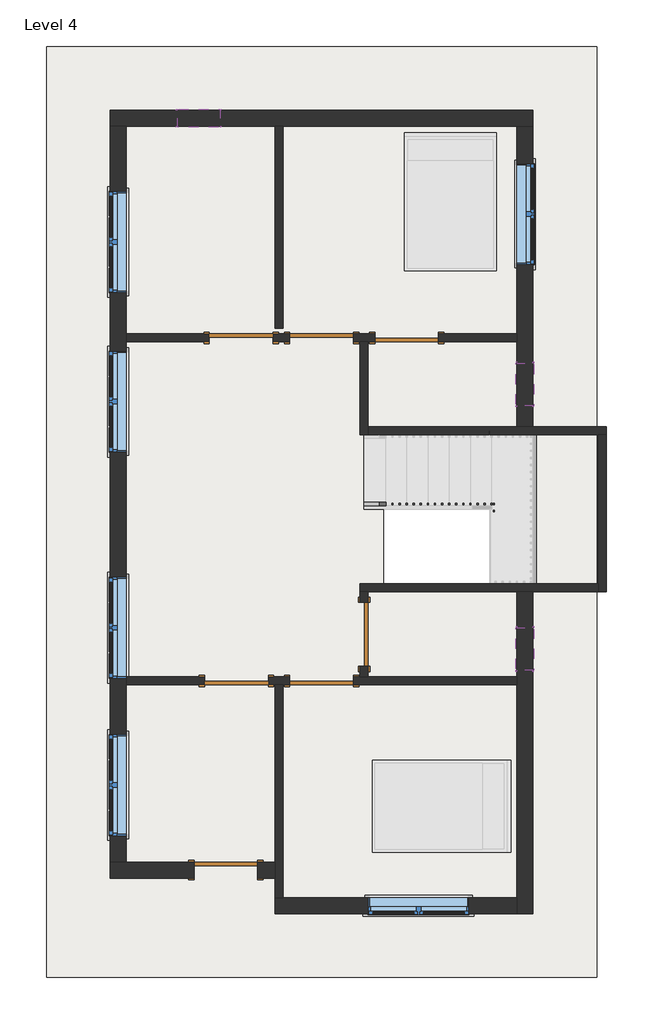
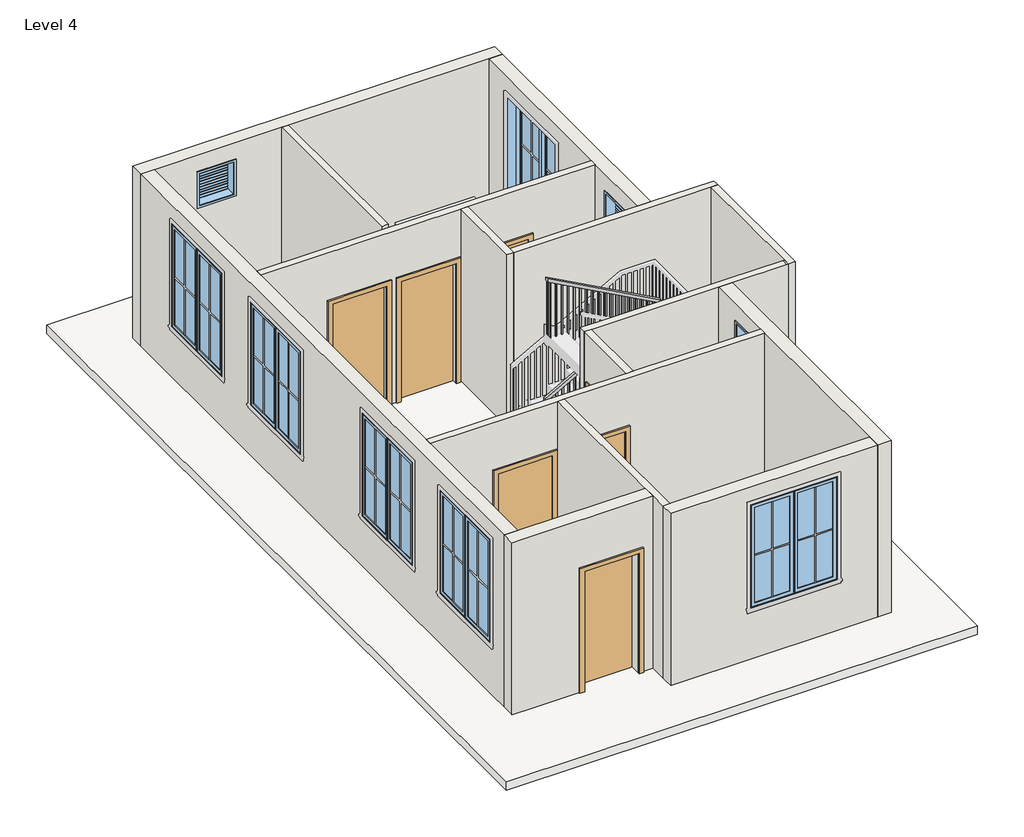
# One storey, part 1 of 2: 15 walls, 9 windows, 7 doors, 1 railing, 1 roof.
"""IFC4 building model written with IfcOpenShell, lengths in millimetres."""

from ifc_helpers import new_model, si_unit, frame, origin, place, context, project, spatial, polyline, outline, extrude, faceted_brep, transform, mapped, element, save
from components import door_e5f9f3c4, door_305aa2a5, door_0ca8825f, window_9ac97e1a, window_f2d8fef0

model = new_model("IFC4")

# Units and contexts
model_context = context("Model", 3, world=origin())
ifc_project = project(units=[si_unit("LENGTHUNIT", "METRE", prefix="MILLI")], contexts=[model_context])

# Site, building, storey
site = spatial("IfcSite", under=ifc_project)
building = spatial("IfcBuilding", under=site)
storey = spatial("IfcBuildingStorey", under=building, Name="Level 4", Elevation=6400.8)

# Doors
placement = place(None, origin())
door_shape = door_e5f9f3c4(model_context)
element("IfcDoor", 1, ObjectType="Single-Flush : 36\" x 84\"", at=placement, inside=storey, context=model_context, shape_type="MappedRepresentation", body=[
    mapped(door_shape, transform((-2929.7888307, 2238.9017201, 6400.8), x_axis=(1.0, 0.0, 0.0), y_axis=(0.0, 1.0, 0.0), z_axis=(0.0, 0.0, 1.0))),
])
element("IfcDoor", 2, ObjectType="Single-Flush : 36\" x 84\"", at=placement, inside=storey, context=model_context, shape_type="MappedRepresentation", body=[
    mapped(door_shape, transform((-558.0638307, 2238.9017201, 6400.8), x_axis=(-1.0, 0.0, 0.0), y_axis=(0.0, -1.0, 0.0), z_axis=(0.0, 0.0, 1.0))),
])
element("IfcDoor", 3, ObjectType="Single-Flush : 36\" x 84\"", at=placement, inside=storey, context=model_context, shape_type="MappedRepresentation", body=[
    mapped(door_shape, transform((-1167.6638307, -2009.2482799, 6400.8), x_axis=(0.0, -1.0, 0.0), y_axis=(1.0, 0.0, 0.0), z_axis=(0.0, 0.0, 1.0))),
])
element("IfcDoor", 4, ObjectType="Single-Flush : 36\" x 84\"", at=placement, inside=storey, context=model_context, shape_type="MappedRepresentation", body=[
    mapped(door_shape, transform((-1777.2638307, -2675.9982799, 6400.8), x_axis=(-1.0, 0.0, 0.0), y_axis=(0.0, -1.0, 0.0), z_axis=(0.0, 0.0, 1.0))),
])
door_2_shape = door_305aa2a5(model_context)
element("IfcDoor", 5, ObjectType="Single-Flush : 36\" x 84\"", at=placement, inside=storey, context=model_context, shape_type="MappedRepresentation", body=[
    mapped(door_2_shape, transform((-1777.2638307, 2238.9017201, 6400.8), x_axis=(-1.0, 0.0, 0.0), y_axis=(0.0, -1.0, 0.0), z_axis=(0.0, 0.0, 1.0))),
])
element("IfcDoor", 6, ObjectType="Single-Flush : 36\" x 84\"", at=placement, inside=storey, context=model_context, shape_type="MappedRepresentation", body=[
    mapped(door_2_shape, transform((-2996.4638307, -2675.9982799, 6400.8), x_axis=(1.0, 0.0, 0.0), y_axis=(0.0, 1.0, 0.0), z_axis=(0.0, 0.0, 1.0))),
])
door_3_shape = door_0ca8825f(model_context)
element("IfcDoor", 7, ObjectType="Single-Flush : 36\" x 84\"", at=placement, inside=storey, context=model_context, shape_type="MappedRepresentation", body=[
    mapped(door_3_shape, transform((-3148.8638307, -5387.4482799, 6400.8), x_axis=(1.0, 0.0, 0.0), y_axis=(0.0, 1.0, 0.0), z_axis=(0.0, 0.0, 1.0))),
])

# Railing
element("IfcRailing", 8, ObjectType="Handrail - Rectangular", at=placement, inside=storey, context=model_context, shape_type="SolidModel", body=[
    faceted_brep([(-1167.6638307, -116.9482799, 7484.5333333), (-1167.6638307, -116.9482799, 7426.4675836), (-1167.6638307, -167.7482799, 7426.4675836), (-1167.6638307, -167.7482799, 7484.5333333), (591.2861693, -116.9482799, 8458.3464821), (642.0861693, -116.9482799, 8428.4052998), (642.0861693, -167.7482799, 8428.4052998), (591.2861693, -167.7482799, 8458.3464821), (591.2861693, -116.9482799, 8500.5333333), (642.0861693, -116.9482799, 8449.7333333), (642.0861693, -167.7482799, 8449.7333333), (591.2861693, -167.7482799, 8500.5333333), (718.2861693, -116.9482799, 8500.5333333), (718.2861693, -116.9482799, 8449.7333333), (667.4861693, -167.7482799, 8449.7333333), (667.4861693, -167.7482799, 8500.5333333), (718.2861693, -218.5482799, 8500.5333333), (667.4861693, -218.5482799, 8500.5333333), (667.4861693, -269.3482799, 8449.7333333), (718.2861693, -269.3482799, 8449.7333333)], [[[0, 1, 2, 3]], [[1, 0, 4, 5]], [[2, 1, 5, 6]], [[3, 2, 6, 7]], [[0, 3, 7, 4]], [[5, 4, 8, 9]], [[6, 5, 9, 10]], [[7, 6, 10, 11]], [[4, 7, 11, 8]], [[9, 8, 12, 13]], [[10, 9, 13, 14]], [[11, 10, 14, 15]], [[8, 11, 15, 12]], [[16, 17, 18, 19]], [[13, 12, 16, 19]], [[14, 13, 19, 18]], [[15, 14, 18, 17]], [[12, 15, 17, 16]]]),
    faceted_brep([(718.2861693, -218.5482799, 8500.5333333), (718.2861693, -269.3482799, 8449.7333333), (667.4861693, -269.3482799, 8449.7333333), (667.4861693, -218.5482799, 8500.5333333), (718.2861693, -218.5482799, 8642.0310502), (667.4861693, -218.5482799, 8611.9403208), (667.4861693, -269.3482799, 8611.9403208), (718.2861693, -269.3482799, 8642.0310502)], [[[0, 1, 2, 3]], [[4, 5, 6, 7]], [[1, 0, 4, 7]], [[2, 1, 7, 6]], [[3, 2, 6, 5]], [[0, 3, 5, 4]]]),
    faceted_brep([(718.2861693, -269.3482799, 8642.0310502), (667.4861693, -269.3482799, 8611.9403208), (667.4861693, -218.5482799, 8611.9403208), (718.2861693, -218.5482799, 8642.0310502), (-1186.7138307, -269.3482799, 9685.8666667), (-1186.7138307, -218.5482799, 9685.8666667), (-1186.7138307, -218.5482799, 9627.9403208), (-1186.7138307, -269.3482799, 9627.9403208)], [[[0, 1, 2, 3]], [[4, 5, 6, 7]], [[1, 0, 4, 7]], [[2, 1, 7, 6]], [[3, 2, 6, 5]], [[0, 3, 5, 4]]]),
    extrude(outline(polyline([(9594.8855263, -1126.3888307), (9605.3238825, -1145.4388307), (8602.1333333, -1145.4388307), (8602.1333333, -1126.3888307), (9594.8855263, -1126.3888307)])), frame((0.0, -253.4732799, 0.0), z_axis=(0.0, 1.0, 0.0), x_axis=(0.0, 0.0, 1.0)), (0.0, 0.0, 1.0), 19.05),
    extrude(outline(polyline([(9539.2142934, -1024.7888307), (9549.6526496, -1043.8388307), (8602.1333333, -1043.8388307), (8602.1333333, -1024.7888307), (9539.2142934, -1024.7888307)])), frame((0.0, -253.4732799, 0.0), z_axis=(0.0, 1.0, 0.0), x_axis=(0.0, 0.0, 1.0)), (0.0, 0.0, 1.0), 19.05),
    extrude(outline(polyline([(9483.5430606, -923.1888307), (9493.9814167, -942.2388307), (8602.1333333, -942.2388307), (8602.1333333, -923.1888307), (9483.5430606, -923.1888307)])), frame((0.0, -253.4732799, 0.0), z_axis=(0.0, 1.0, 0.0), x_axis=(0.0, 0.0, 1.0)), (0.0, 0.0, 1.0), 19.05),
    extrude(outline(polyline([(9427.8718277, -821.5888307), (9438.3101838, -840.6388307), (8432.8, -840.6388307), (8432.8, -821.5888307), (9427.8718277, -821.5888307)])), frame((0.0, -253.4732799, 0.0), z_axis=(0.0, 1.0, 0.0), x_axis=(0.0, 0.0, 1.0)), (0.0, 0.0, 1.0), 19.05),
    extrude(outline(polyline([(9372.2005948, -719.9888307), (9382.638951, -739.0388307), (8432.8, -739.0388307), (8432.8, -719.9888307), (9372.2005948, -719.9888307)])), frame((0.0, -253.4732799, 0.0), z_axis=(0.0, 1.0, 0.0), x_axis=(0.0, 0.0, 1.0)), (0.0, 0.0, 1.0), 19.05),
    extrude(outline(polyline([(9316.5293619, -618.3888307), (9326.9677181, -637.4388307), (8432.8, -637.4388307), (8432.8, -618.3888307), (9316.5293619, -618.3888307)])), frame((0.0, -253.4732799, 0.0), z_axis=(0.0, 1.0, 0.0), x_axis=(0.0, 0.0, 1.0)), (0.0, 0.0, 1.0), 19.05),
    extrude(outline(polyline([(9260.858129, -516.7888307), (9271.2964852, -535.8388307), (8263.4666667, -535.8388307), (8263.4666667, -516.7888307), (9260.858129, -516.7888307)])), frame((0.0, -253.4732799, 0.0), z_axis=(0.0, 1.0, 0.0), x_axis=(0.0, 0.0, 1.0)), (0.0, 0.0, 1.0), 19.05),
    extrude(outline(polyline([(9205.1868962, -415.1888307), (9215.6252523, -434.2388307), (8263.4666667, -434.2388307), (8263.4666667, -415.1888307), (9205.1868962, -415.1888307)])), frame((0.0, -253.4732799, 0.0), z_axis=(0.0, 1.0, 0.0), x_axis=(0.0, 0.0, 1.0)), (0.0, 0.0, 1.0), 19.05),
    extrude(outline(polyline([(9149.5156633, -313.5888307), (9159.9540195, -332.6388307), (8263.4666667, -332.6388307), (8263.4666667, -313.5888307), (9149.5156633, -313.5888307)])), frame((0.0, -253.4732799, 0.0), z_axis=(0.0, 1.0, 0.0), x_axis=(0.0, 0.0, 1.0)), (0.0, 0.0, 1.0), 19.05),
    extrude(outline(polyline([(9093.8444304, -211.9888307), (9104.2827866, -231.0388307), (8094.1333333, -231.0388307), (8094.1333333, -211.9888307), (9093.8444304, -211.9888307)])), frame((0.0, -253.4732799, 0.0), z_axis=(0.0, 1.0, 0.0), x_axis=(0.0, 0.0, 1.0)), (0.0, 0.0, 1.0), 19.05),
    extrude(outline(polyline([(9038.1731975, -110.3888307), (9048.6115537, -129.4388307), (8094.1333333, -129.4388307), (8094.1333333, -110.3888307), (9038.1731975, -110.3888307)])), frame((0.0, -253.4732799, 0.0), z_axis=(0.0, 1.0, 0.0), x_axis=(0.0, 0.0, 1.0)), (0.0, 0.0, 1.0), 19.05),
    extrude(outline(polyline([(8982.5019647, -8.7888307), (8992.9403208, -27.8388307), (8094.1333333, -27.8388307), (8094.1333333, -8.7888307), (8982.5019647, -8.7888307)])), frame((0.0, -253.4732799, 0.0), z_axis=(0.0, 1.0, 0.0), x_axis=(0.0, 0.0, 1.0)), (0.0, 0.0, 1.0), 19.05),
    extrude(outline(polyline([(8926.8307318, 92.8111693), (8937.2690879, 73.7611693), (7924.8, 73.7611693), (7924.8, 92.8111693), (8926.8307318, 92.8111693)])), frame((0.0, -253.4732799, 0.0), z_axis=(0.0, 1.0, 0.0), x_axis=(0.0, 0.0, 1.0)), (0.0, 0.0, 1.0), 19.05),
    extrude(outline(polyline([(8871.1594989, 194.4111693), (8881.5978551, 175.3611693), (7924.8, 175.3611693), (7924.8, 194.4111693), (8871.1594989, 194.4111693)])), frame((0.0, -253.4732799, 0.0), z_axis=(0.0, 1.0, 0.0), x_axis=(0.0, 0.0, 1.0)), (0.0, 0.0, 1.0), 19.05),
    extrude(outline(polyline([(8815.488266, 296.0111693), (8825.9266222, 276.9611693), (7924.8, 276.9611693), (7924.8, 296.0111693), (8815.488266, 296.0111693)])), frame((0.0, -253.4732799, 0.0), z_axis=(0.0, 1.0, 0.0), x_axis=(0.0, 0.0, 1.0)), (0.0, 0.0, 1.0), 19.05),
    extrude(outline(polyline([(8759.8170332, 397.6111693), (8770.2553893, 378.5611693), (7755.4666667, 378.5611693), (7755.4666667, 397.6111693), (8759.8170332, 397.6111693)])), frame((0.0, -253.4732799, 0.0), z_axis=(0.0, 1.0, 0.0), x_axis=(0.0, 0.0, 1.0)), (0.0, 0.0, 1.0), 19.05),
    extrude(outline(polyline([(8704.1458003, 499.2111693), (8714.5841564, 480.1611693), (7755.4666667, 480.1611693), (7755.4666667, 499.2111693), (8704.1458003, 499.2111693)])), frame((0.0, -253.4732799, 0.0), z_axis=(0.0, 1.0, 0.0), x_axis=(0.0, 0.0, 1.0)), (0.0, 0.0, 1.0), 19.05),
    extrude(outline(polyline([(8648.4745674, 600.8111693), (8658.9129236, 581.7611693), (7755.4666667, 581.7611693), (7755.4666667, 600.8111693), (8648.4745674, 600.8111693)])), frame((0.0, -253.4732799, 0.0), z_axis=(0.0, 1.0, 0.0), x_axis=(0.0, 0.0, 1.0)), (0.0, 0.0, 1.0), 19.05),
    extrude(outline(polyline([(651.6111693, -151.8732799), (651.6111693, -132.8232799), (670.6611693, -132.8232799), (670.6611693, -151.8732799), (651.6111693, -151.8732799)])), frame((0.0, 0.0, 7416.8), z_axis=(0.0, 0.0, 1.0), x_axis=(1.0, 0.0, 0.0)), (0.0, 0.0, 1.0), 1032.9333333),
    extrude(outline(polyline([(8387.9762341, 569.0611693), (8377.4295213, 550.0111693), (7416.8, 550.0111693), (7416.8, 569.0611693), (8387.9762341, 569.0611693)])), frame((0.0, -151.8732799, 0.0), z_axis=(0.0, 1.0, 0.0), x_axis=(0.0, 0.0, 1.0)), (0.0, 0.0, 1.0), 19.05),
    extrude(outline(polyline([(8331.7270991, 467.4611693), (8321.1803863, 448.4111693), (7416.8, 448.4111693), (7416.8, 467.4611693), (8331.7270991, 467.4611693)])), frame((0.0, -151.8732799, 0.0), z_axis=(0.0, 1.0, 0.0), x_axis=(0.0, 0.0, 1.0)), (0.0, 0.0, 1.0), 19.05),
    extrude(outline(polyline([(8275.4779642, 365.8611693), (8264.9312514, 346.8111693), (7247.4666667, 346.8111693), (7247.4666667, 365.8611693), (8275.4779642, 365.8611693)])), frame((0.0, -151.8732799, 0.0), z_axis=(0.0, 1.0, 0.0), x_axis=(0.0, 0.0, 1.0)), (0.0, 0.0, 1.0), 19.05),
    extrude(outline(polyline([(8219.2288292, 264.2611693), (8208.6821164, 245.2111693), (7247.4666667, 245.2111693), (7247.4666667, 264.2611693), (8219.2288292, 264.2611693)])), frame((0.0, -151.8732799, 0.0), z_axis=(0.0, 1.0, 0.0), x_axis=(0.0, 0.0, 1.0)), (0.0, 0.0, 1.0), 19.05),
    extrude(outline(polyline([(8162.9796943, 162.6611693), (8152.4329815, 143.6111693), (7247.4666667, 143.6111693), (7247.4666667, 162.6611693), (8162.9796943, 162.6611693)])), frame((0.0, -151.8732799, 0.0), z_axis=(0.0, 1.0, 0.0), x_axis=(0.0, 0.0, 1.0)), (0.0, 0.0, 1.0), 19.05),
    extrude(outline(polyline([(8106.7305593, 61.0611693), (8096.1838465, 42.0111693), (7078.1333333, 42.0111693), (7078.1333333, 61.0611693), (8106.7305593, 61.0611693)])), frame((0.0, -151.8732799, 0.0), z_axis=(0.0, 1.0, 0.0), x_axis=(0.0, 0.0, 1.0)), (0.0, 0.0, 1.0), 19.05),
    extrude(outline(polyline([(8050.4814244, -40.5388307), (8039.9347116, -59.5888307), (7078.1333333, -59.5888307), (7078.1333333, -40.5388307), (8050.4814244, -40.5388307)])), frame((0.0, -151.8732799, 0.0), z_axis=(0.0, 1.0, 0.0), x_axis=(0.0, 0.0, 1.0)), (0.0, 0.0, 1.0), 19.05),
    extrude(outline(polyline([(7994.2322895, -142.1388307), (7983.6855766, -161.1888307), (7078.1333333, -161.1888307), (7078.1333333, -142.1388307), (7994.2322895, -142.1388307)])), frame((0.0, -151.8732799, 0.0), z_axis=(0.0, 1.0, 0.0), x_axis=(0.0, 0.0, 1.0)), (0.0, 0.0, 1.0), 19.05),
    extrude(outline(polyline([(7937.9831545, -243.7388307), (7927.4364417, -262.7888307), (6908.8, -262.7888307), (6908.8, -243.7388307), (7937.9831545, -243.7388307)])), frame((0.0, -151.8732799, 0.0), z_axis=(0.0, 1.0, 0.0), x_axis=(0.0, 0.0, 1.0)), (0.0, 0.0, 1.0), 19.05),
    extrude(outline(polyline([(7881.7340196, -345.3388307), (7871.1873068, -364.3888307), (6908.8, -364.3888307), (6908.8, -345.3388307), (7881.7340196, -345.3388307)])), frame((0.0, -151.8732799, 0.0), z_axis=(0.0, 1.0, 0.0), x_axis=(0.0, 0.0, 1.0)), (0.0, 0.0, 1.0), 19.05),
    extrude(outline(polyline([(7825.4848846, -446.9388307), (7814.9381718, -465.9888307), (6908.8, -465.9888307), (6908.8, -446.9388307), (7825.4848846, -446.9388307)])), frame((0.0, -151.8732799, 0.0), z_axis=(0.0, 1.0, 0.0), x_axis=(0.0, 0.0, 1.0)), (0.0, 0.0, 1.0), 19.05),
    extrude(outline(polyline([(7769.2357497, -548.5388307), (7758.6890369, -567.5888307), (6739.4666667, -567.5888307), (6739.4666667, -548.5388307), (7769.2357497, -548.5388307)])), frame((0.0, -151.8732799, 0.0), z_axis=(0.0, 1.0, 0.0), x_axis=(0.0, 0.0, 1.0)), (0.0, 0.0, 1.0), 19.05),
    extrude(outline(polyline([(7712.9866147, -650.1388307), (7702.4399019, -669.1888307), (6739.4666667, -669.1888307), (6739.4666667, -650.1388307), (7712.9866147, -650.1388307)])), frame((0.0, -151.8732799, 0.0), z_axis=(0.0, 1.0, 0.0), x_axis=(0.0, 0.0, 1.0)), (0.0, 0.0, 1.0), 19.05),
    extrude(outline(polyline([(7656.7374798, -751.7388307), (7646.190767, -770.7888307), (6739.4666667, -770.7888307), (6739.4666667, -751.7388307), (7656.7374798, -751.7388307)])), frame((0.0, -151.8732799, 0.0), z_axis=(0.0, 1.0, 0.0), x_axis=(0.0, 0.0, 1.0)), (0.0, 0.0, 1.0), 19.05),
    extrude(outline(polyline([(7600.4883448, -853.3388307), (7589.941632, -872.3888307), (6570.1333333, -872.3888307), (6570.1333333, -853.3388307), (7600.4883448, -853.3388307)])), frame((0.0, -151.8732799, 0.0), z_axis=(0.0, 1.0, 0.0), x_axis=(0.0, 0.0, 1.0)), (0.0, 0.0, 1.0), 19.05),
    extrude(outline(polyline([(7544.2392099, -954.9388307), (7533.6924971, -973.9888307), (6570.1333333, -973.9888307), (6570.1333333, -954.9388307), (7544.2392099, -954.9388307)])), frame((0.0, -151.8732799, 0.0), z_axis=(0.0, 1.0, 0.0), x_axis=(0.0, 0.0, 1.0)), (0.0, 0.0, 1.0), 19.05),
    extrude(outline(polyline([(7487.9900749, -1056.5388307), (7477.4433621, -1075.5888307), (6570.1333333, -1075.5888307), (6570.1333333, -1056.5388307), (7487.9900749, -1056.5388307)])), frame((0.0, -151.8732799, 0.0), z_axis=(0.0, 1.0, 0.0), x_axis=(0.0, 0.0, 1.0)), (0.0, 0.0, 1.0), 19.05),
    extrude(outline(polyline([(683.3611693, -234.4232799), (702.4111693, -234.4232799), (702.4111693, -253.4732799), (683.3611693, -253.4732799), (683.3611693, -234.4232799)])), frame((0.0, 0.0, 7586.1333333), z_axis=(0.0, 0.0, 1.0), x_axis=(1.0, 0.0, 0.0)), (0.0, 0.0, 1.0), 863.6),
    extrude(outline(polyline([(683.3611693, -151.8732799), (683.3611693, -132.8232799), (702.4111693, -132.8232799), (702.4111693, -151.8732799), (683.3611693, -151.8732799)])), frame((0.0, 0.0, 7586.1333333), z_axis=(0.0, 0.0, 1.0), x_axis=(1.0, 0.0, 0.0)), (0.0, 0.0, 1.0), 863.6),
    extrude(outline(polyline([(9617.5019647, -1167.6638307), (9627.9403208, -1186.7138307), (8602.1333333, -1186.7138307), (8602.1333333, -1167.6638307), (9617.5019647, -1167.6638307)])), frame((0.0, -253.4732799, 0.0), z_axis=(0.0, 1.0, 0.0), x_axis=(0.0, 0.0, 1.0)), (0.0, 0.0, 1.0), 19.05),
    extrude(outline(polyline([(7437.0142964, -1148.6138307), (7426.4675836, -1167.6638307), (6570.1333333, -1167.6638307), (6570.1333333, -1148.6138307), (7437.0142964, -1148.6138307)])), frame((0.0, -151.8732799, 0.0), z_axis=(0.0, 1.0, 0.0), x_axis=(0.0, 0.0, 1.0)), (0.0, 0.0, 1.0), 19.05),
])

# Roof
element("IfcRoof", 9, ObjectType="ROOF 6\"", at=placement, inside=storey, context=model_context, shape_type="SweptSolid", body=[
    extrude(outline(polyline([(-5720.6138307, -6924.1482799), (-5720.6138307, 6410.8517201), (2166.0861693, 6410.8517201), (2166.0861693, -6924.1482799), (-5720.6138307, -6924.1482799)]), holes=[polyline([(1251.6861693, -1285.3482799), (1251.6861693, 899.0517201), (-881.9138307, 899.0517201), (-881.9138307, -1285.3482799), (1251.6861693, -1285.3482799)])]), frame((0.0, 0.0, 6248.4), z_axis=(0.0, 0.0, 1.0), x_axis=(1.0, 0.0, 0.0)), (0.0, 0.0, 1.0), 152.4),
])

# Walls
element("IfcWall", 10, ObjectType="WALL 4.5\"", at=placement, inside=storey, context=model_context, shape_type="SweptSolid", body=[
    extrude(outline(polyline([(-2444.0138307, 2372.2517201), (-2444.0138307, 5267.8517201), (-2329.7138307, 5267.8517201), (-2329.7138307, 2372.2517201), (-2444.0138307, 2372.2517201)])), frame((0.0, 0.0, 6400.8), z_axis=(0.0, 0.0, 1.0), x_axis=(1.0, 0.0, 0.0)), (0.0, 0.0, 1.0), 3048.0),
])
element("IfcWall", 11, ObjectType="WALL 4.5\"", at=placement, inside=storey, context=model_context, shape_type="Brep", body=[
    faceted_brep([(-1320.0638307, 2181.7517201, 6400.8), (-1224.8138307, 2181.7517201, 6400.8), (-1110.5138307, 2181.7517201, 6400.8), (-1015.2638307, 2181.7517201, 6400.8), (-1015.2638307, 2181.7517201, 8534.4), (-100.8638307, 2181.7517201, 8534.4), (-100.8638307, 2181.7517201, 6400.8), (1023.0861693, 2181.7517201, 6400.8), (1023.0861693, 2181.7517201, 9448.8), (-1110.5138307, 2181.7517201, 9448.8), (-1224.8138307, 2181.7517201, 9448.8), (-4577.6138307, 2181.7517201, 9448.8), (-4577.6138307, 2181.7517201, 6400.8), (-3386.9888307, 2181.7517201, 6400.8), (-3386.9888307, 2181.7517201, 8534.4), (-2472.5888307, 2181.7517201, 8534.4), (-2472.5888307, 2181.7517201, 6400.8), (-2234.4638307, 2181.7517201, 6400.8), (-2234.4638307, 2181.7517201, 8534.4), (-1320.0638307, 2181.7517201, 8534.4), (-1015.2638307, 2296.0517201, 8534.4), (-1015.2638307, 2296.0517201, 6400.8), (-1320.0638307, 2296.0517201, 6400.8), (-1320.0638307, 2296.0517201, 8534.4), (-2234.4638307, 2296.0517201, 8534.4), (-2234.4638307, 2296.0517201, 6400.8), (-2472.5888307, 2296.0517201, 6400.8), (-2472.5888307, 2296.0517201, 8534.4), (-3386.9888307, 2296.0517201, 8534.4), (-3386.9888307, 2296.0517201, 6400.8), (-4577.6138307, 2296.0517201, 6400.8), (-4577.6138307, 2296.0517201, 9448.8), (1023.0861693, 2296.0517201, 9448.8), (1023.0861693, 2296.0517201, 6400.8), (-100.8638307, 2296.0517201, 6400.8), (-100.8638307, 2296.0517201, 8534.4)], [[[0, 1, 2, 3, 4, 5, 6, 7, 8, 9, 10, 11, 12, 13, 14, 15, 16, 17, 18, 19]], [[20, 21, 22, 23, 24, 25, 26, 27, 28, 29, 30, 31, 32, 33, 34, 35]], [[13, 12, 30, 29]], [[26, 25, 17, 16]], [[34, 33, 7, 6]], [[22, 21, 3, 2, 1, 0]], [[8, 7, 33, 32]], [[12, 11, 31, 30]], [[27, 26, 16, 15]], [[28, 27, 15, 14]], [[29, 28, 14, 13]], [[18, 17, 25, 24]], [[19, 18, 24, 23]], [[0, 19, 23, 22]], [[4, 3, 21, 20]], [[5, 4, 20, 35]], [[6, 5, 35, 34]], [[11, 10, 9, 8, 32, 31]]]),
])
element("IfcWall", 12, ObjectType="WALL 4.5\"", at=placement, inside=storey, context=model_context, shape_type="Brep", body=[
    faceted_brep([(-1224.8138307, 2181.7517201, 6400.8), (-1224.8138307, 848.2517201, 6400.8), (-1224.8138307, 848.2517201, 9448.8), (-1224.8138307, 2181.7517201, 9448.8), (-1110.5138307, 2181.7517201, 6400.8), (-1110.5138307, 2181.7517201, 9448.8), (-1110.5138307, 962.5517201, 9448.8), (-1110.5138307, 848.2517201, 9448.8), (-1110.5138307, 848.2517201, 6400.8), (-1110.5138307, 962.5517201, 6400.8)], [[[0, 1, 2, 3]], [[4, 5, 6, 7, 8, 9]], [[1, 0, 4, 9, 8]], [[0, 3, 5, 4]], [[2, 1, 8, 7]], [[3, 2, 7, 6, 5]]]),
])
element("IfcWall", 13, ObjectType="WALL 4.5\"", at=placement, inside=storey, context=model_context, shape_type="Brep", body=[
    faceted_brep([(-1110.5138307, 848.2517201, 6400.8), (2191.4861693, 848.2517201, 6400.8), (2305.7861693, 848.2517201, 6400.8), (2305.7861693, 848.2517201, 9448.8), (2191.4861693, 848.2517201, 9448.8), (-1110.5138307, 848.2517201, 9448.8), (-1110.5138307, 962.5517201, 6400.8), (-1110.5138307, 962.5517201, 9448.8), (1023.0861693, 962.5517201, 9448.8), (1251.6861693, 962.5517201, 9448.8), (2305.7861693, 962.5517201, 9448.8), (2305.7861693, 962.5517201, 6400.8), (1251.6861693, 962.5517201, 6400.8), (1023.0861693, 962.5517201, 6400.8)], [[[0, 1, 2, 3, 4, 5]], [[6, 7, 8, 9, 10, 11, 12, 13]], [[2, 1, 0, 6, 13, 12, 11]], [[5, 4, 3, 10, 9, 8, 7]], [[0, 5, 7, 6]], [[3, 2, 11, 10]]]),
])
element("IfcWall", 14, ObjectType="WALL 4.5\"", at=placement, inside=storey, context=model_context, shape_type="Brep", body=[
    faceted_brep([(2191.4861693, 848.2517201, 6400.8), (2191.4861693, -1285.3482799, 6400.8), (2191.4861693, -1399.6482799, 6400.8), (2191.4861693, -1399.6482799, 9448.8), (2191.4861693, -1285.3482799, 9448.8), (2191.4861693, 848.2517201, 9448.8), (2305.7861693, 848.2517201, 6400.8), (2305.7861693, 848.2517201, 9448.8), (2305.7861693, -1399.6482799, 9448.8), (2305.7861693, -1399.6482799, 6400.8)], [[[0, 1, 2, 3, 4, 5]], [[6, 7, 8, 9]], [[2, 1, 0, 6, 9]], [[5, 4, 3, 8, 7]], [[0, 5, 7, 6]], [[3, 2, 9, 8]]]),
])
element("IfcWall", 15, ObjectType="WALL 4.5\"", at=placement, inside=storey, context=model_context, shape_type="Brep", body=[
    faceted_brep([(2191.4861693, -1285.3482799, 6400.8), (-1224.8138307, -1285.3482799, 6400.8), (-1224.8138307, -1285.3482799, 9448.8), (-881.9138307, -1285.3482799, 9448.8), (1251.6861693, -1285.3482799, 9448.8), (2166.0861693, -1285.3482799, 9448.8), (2191.4861693, -1285.3482799, 9448.8), (2191.4861693, -1399.6482799, 6400.8), (2191.4861693, -1399.6482799, 9448.8), (2166.0861693, -1399.6482799, 9448.8), (1251.6861693, -1399.6482799, 9448.8), (1023.0861693, -1399.6482799, 9448.8), (-1110.5138307, -1399.6482799, 9448.8), (-1224.8138307, -1399.6482799, 9448.8), (-1224.8138307, -1399.6482799, 6400.8), (-1110.5138307, -1399.6482799, 6400.8), (1023.0861693, -1399.6482799, 6400.8), (1251.6861693, -1399.6482799, 6400.8)], [[[0, 1, 2, 3, 4, 5, 6]], [[7, 8, 9, 10, 11, 12, 13, 14, 15, 16, 17]], [[1, 0, 7, 17, 16, 15, 14]], [[0, 6, 8, 7]], [[2, 1, 14, 13]], [[6, 5, 9, 8]], [[5, 4, 3, 2, 13, 12, 11, 10, 9]]]),
])
element("IfcWall", 16, ObjectType="WALL 4.5\"", at=placement, inside=storey, context=model_context, shape_type="SweptSolid", body=[
    extrude(outline(polyline([(-2466.4482799, 8534.4), (-2466.4482799, 6400.8), (-2618.8482799, 6400.8), (-2618.8482799, 9448.8), (-1399.6482799, 9448.8), (-1399.6482799, 6400.8), (-1552.0482799, 6400.8), (-1552.0482799, 8534.4), (-2466.4482799, 8534.4)])), frame((-1224.8138307, 0.0, 0.0), z_axis=(1.0, 0.0, 0.0), x_axis=(0.0, 1.0, 0.0)), (0.0, 0.0, 1.0), 114.3),
])
element("IfcWall", 17, ObjectType="WALL 4.5\"", at=placement, inside=storey, context=model_context, shape_type="Brep", body=[
    faceted_brep([(-2234.4638307, -2618.8482799, 6400.8), (-2539.2638307, -2618.8482799, 6400.8), (-2539.2638307, -2618.8482799, 8534.4), (-3453.6638307, -2618.8482799, 8534.4), (-3453.6638307, -2618.8482799, 6400.8), (-4577.6138307, -2618.8482799, 6400.8), (-4577.6138307, -2618.8482799, 9448.8), (-1224.8138307, -2618.8482799, 9448.8), (-1110.5138307, -2618.8482799, 9448.8), (1023.0861693, -2618.8482799, 9448.8), (1023.0861693, -2618.8482799, 6400.8), (-1110.5138307, -2618.8482799, 6400.8), (-1224.8138307, -2618.8482799, 6400.8), (-1320.0638307, -2618.8482799, 6400.8), (-1320.0638307, -2618.8482799, 8534.4), (-2234.4638307, -2618.8482799, 8534.4), (-2539.2638307, -2733.1482799, 8534.4), (-2539.2638307, -2733.1482799, 6400.8), (-2444.0138307, -2733.1482799, 6400.8), (-2329.7138307, -2733.1482799, 6400.8), (-2234.4638307, -2733.1482799, 6400.8), (-2234.4638307, -2733.1482799, 8534.4), (-1320.0638307, -2733.1482799, 8534.4), (-1320.0638307, -2733.1482799, 6400.8), (1023.0861693, -2733.1482799, 6400.8), (1023.0861693, -2733.1482799, 9448.8), (-2329.7138307, -2733.1482799, 9448.8), (-2444.0138307, -2733.1482799, 9448.8), (-4577.6138307, -2733.1482799, 9448.8), (-4577.6138307, -2733.1482799, 6400.8), (-3453.6638307, -2733.1482799, 6400.8), (-3453.6638307, -2733.1482799, 8534.4)], [[[0, 1, 2, 3, 4, 5, 6, 7, 8, 9, 10, 11, 12, 13, 14, 15]], [[16, 17, 18, 19, 20, 21, 22, 23, 24, 25, 26, 27, 28, 29, 30, 31]], [[13, 12, 11, 10, 24, 23]], [[30, 29, 5, 4]], [[20, 19, 18, 17, 1, 0]], [[10, 9, 25, 24]], [[6, 5, 29, 28]], [[21, 20, 0, 15]], [[22, 21, 15, 14]], [[23, 22, 14, 13]], [[2, 1, 17, 16]], [[3, 2, 16, 31]], [[4, 3, 31, 30]], [[9, 8, 7, 6, 28, 27, 26, 25]]]),
])
element("IfcWall", 18, ObjectType="WALL 4.5\"", at=placement, inside=storey, context=model_context, shape_type="Brep", body=[
    faceted_brep([(-2329.7138307, -5781.1482799, 6400.8), (-2329.7138307, -2733.1482799, 6400.8), (-2329.7138307, -2733.1482799, 9448.8), (-2329.7138307, -5781.1482799, 9448.8), (-2444.0138307, -5781.1482799, 6400.8), (-2444.0138307, -5781.1482799, 9448.8), (-2444.0138307, -5501.7482799, 9448.8), (-2444.0138307, -5273.1482799, 9448.8), (-2444.0138307, -2733.1482799, 9448.8), (-2444.0138307, -2733.1482799, 6400.8), (-2444.0138307, -5273.1482799, 6400.8), (-2444.0138307, -5501.7482799, 6400.8)], [[[0, 1, 2, 3]], [[4, 5, 6, 7, 8, 9, 10, 11]], [[1, 0, 4, 11, 10, 9]], [[0, 3, 5, 4]], [[2, 1, 9, 8]], [[3, 2, 8, 7, 6, 5]]]),
])
element("IfcWall", 19, ObjectType="WALL 9\"", at=placement, inside=storey, context=model_context, shape_type="Brep", body=[
    faceted_brep([(-4806.2138307, 5267.8517201, 6400.8), (-4577.6138307, 5267.8517201, 6400.8), (-2444.0138307, 5267.8517201, 6400.8), (-2329.7138307, 5267.8517201, 6400.8), (1023.0861693, 5267.8517201, 6400.8), (1251.6861693, 5267.8517201, 6400.8), (1251.6861693, 5267.8517201, 9448.8), (1023.0861693, 5267.8517201, 9448.8), (-2329.7138307, 5267.8517201, 9448.8), (-2444.0138307, 5267.8517201, 9448.8), (-4577.6138307, 5267.8517201, 9448.8), (-4806.2138307, 5267.8517201, 9448.8), (-3844.1888307, 5267.8517201, 9144.0), (-3234.5888307, 5267.8517201, 9144.0), (-3234.5888307, 5267.8517201, 8534.4), (-3844.1888307, 5267.8517201, 8534.4), (-4806.2138307, 5496.4517201, 6400.8), (-4806.2138307, 5496.4517201, 9448.8), (1251.6861693, 5496.4517201, 9448.8), (1251.6861693, 5496.4517201, 6400.8), (-3844.1888307, 5496.4517201, 9144.0), (-3844.1888307, 5496.4517201, 8534.4), (-3234.5888307, 5496.4517201, 8534.4), (-3234.5888307, 5496.4517201, 9144.0)], [[[0, 1, 2, 3, 4, 5, 6, 7, 8, 9, 10, 11], [12, 13, 14, 15]], [[16, 17, 18, 19], [20, 21, 22, 23]], [[5, 4, 3, 2, 1, 0, 16, 19]], [[6, 5, 19, 18]], [[0, 11, 17, 16]], [[21, 20, 12, 15]], [[22, 21, 15, 14]], [[23, 22, 14, 13]], [[20, 23, 13, 12]], [[11, 10, 9, 8, 7, 6, 18, 17]]]),
])
element("IfcWall", 20, ObjectType="WALL 9\"", at=placement, inside=storey, context=model_context, shape_type="Brep", body=[
    faceted_brep([(1023.0861693, 5267.8517201, 6400.8), (1023.0861693, 2296.0517201, 6400.8), (1023.0861693, 2181.7517201, 6400.8), (1023.0861693, 962.5517201, 6400.8), (1023.0861693, 962.5517201, 9448.8), (1023.0861693, 2181.7517201, 9448.8), (1023.0861693, 2296.0517201, 9448.8), (1023.0861693, 5267.8517201, 9448.8), (1023.0861693, 3286.6517201, 9144.0), (1023.0861693, 3286.6517201, 7315.2), (1023.0861693, 4734.4517201, 7315.2), (1023.0861693, 4734.4517201, 9144.0), (1023.0861693, 1876.9517201, 9144.0), (1023.0861693, 1267.3517201, 9144.0), (1023.0861693, 1267.3517201, 8534.4), (1023.0861693, 1876.9517201, 8534.4), (1251.6861693, 5267.8517201, 6400.8), (1251.6861693, 5267.8517201, 9448.8), (1251.6861693, 962.5517201, 9448.8), (1251.6861693, 962.5517201, 6400.8), (1251.6861693, 3286.6517201, 9144.0), (1251.6861693, 4734.4517201, 9144.0), (1251.6861693, 4734.4517201, 7315.2), (1251.6861693, 3286.6517201, 7315.2), (1251.6861693, 1876.9517201, 9144.0), (1251.6861693, 1876.9517201, 8534.4), (1251.6861693, 1267.3517201, 8534.4), (1251.6861693, 1267.3517201, 9144.0)], [[[0, 1, 2, 3, 4, 5, 6, 7], [8, 9, 10, 11], [12, 13, 14, 15]], [[16, 17, 18, 19], [20, 21, 22, 23], [24, 25, 26, 27]], [[3, 2, 1, 0, 16, 19]], [[0, 7, 17, 16]], [[4, 3, 19, 18]], [[9, 8, 20, 23]], [[10, 9, 23, 22]], [[11, 10, 22, 21]], [[8, 11, 21, 20]], [[25, 24, 12, 15]], [[26, 25, 15, 14]], [[27, 26, 14, 13]], [[24, 27, 13, 12]], [[7, 6, 5, 4, 18, 17]]]),
])
element("IfcWall", 21, ObjectType="WALL 9\"", at=placement, inside=storey, context=model_context, shape_type="Brep", body=[
    faceted_brep([(1023.0861693, -1399.6482799, 6400.8), (1023.0861693, -2618.8482799, 6400.8), (1023.0861693, -2733.1482799, 6400.8), (1023.0861693, -5781.1482799, 6400.8), (1023.0861693, -6009.7482799, 6400.8), (1023.0861693, -6009.7482799, 9448.8), (1023.0861693, -5781.1482799, 9448.8), (1023.0861693, -2733.1482799, 9448.8), (1023.0861693, -2618.8482799, 9448.8), (1023.0861693, -1399.6482799, 9448.8), (1023.0861693, -1913.9982799, 9144.0), (1023.0861693, -2523.5982799, 9144.0), (1023.0861693, -2523.5982799, 8534.4), (1023.0861693, -1913.9982799, 8534.4), (1251.6861693, -1399.6482799, 6400.8), (1251.6861693, -1399.6482799, 9448.8), (1251.6861693, -6009.7482799, 9448.8), (1251.6861693, -6009.7482799, 6400.8), (1251.6861693, -1913.9982799, 9144.0), (1251.6861693, -1913.9982799, 8534.4), (1251.6861693, -2523.5982799, 8534.4), (1251.6861693, -2523.5982799, 9144.0)], [[[0, 1, 2, 3, 4, 5, 6, 7, 8, 9], [10, 11, 12, 13]], [[14, 15, 16, 17], [18, 19, 20, 21]], [[4, 3, 2, 1, 0, 14, 17]], [[5, 4, 17, 16]], [[0, 9, 15, 14]], [[19, 18, 10, 13]], [[20, 19, 13, 12]], [[21, 20, 12, 11]], [[18, 21, 11, 10]], [[9, 8, 7, 6, 5, 16, 15]]]),
])
element("IfcWall", 22, ObjectType="WALL 9\"", at=placement, inside=storey, context=model_context, shape_type="Brep", body=[
    faceted_brep([(1023.0861693, -5781.1482799, 6400.8), (-2329.7138307, -5781.1482799, 6400.8), (-2444.0138307, -5781.1482799, 6400.8), (-2444.0138307, -5781.1482799, 9448.8), (-2329.7138307, -5781.1482799, 9448.8), (1023.0861693, -5781.1482799, 9448.8), (-1110.5138307, -5781.1482799, 9144.0), (-1110.5138307, -5781.1482799, 7315.2), (337.2861693, -5781.1482799, 7315.2), (337.2861693, -5781.1482799, 9144.0), (1023.0861693, -6009.7482799, 6400.8), (1023.0861693, -6009.7482799, 9448.8), (-2444.0138307, -6009.7482799, 9448.8), (-2444.0138307, -6009.7482799, 6400.8), (-1110.5138307, -6009.7482799, 9144.0), (337.2861693, -6009.7482799, 9144.0), (337.2861693, -6009.7482799, 7315.2), (-1110.5138307, -6009.7482799, 7315.2)], [[[0, 1, 2, 3, 4, 5], [6, 7, 8, 9]], [[10, 11, 12, 13], [14, 15, 16, 17]], [[2, 1, 0, 10, 13]], [[0, 5, 11, 10]], [[3, 2, 13, 12]], [[7, 6, 14, 17]], [[8, 7, 17, 16]], [[9, 8, 16, 15]], [[6, 9, 15, 14]], [[5, 4, 3, 12, 11]]]),
])
element("IfcWall", 23, ObjectType="WALL 9\"", at=placement, inside=storey, context=model_context, shape_type="Brep", body=[
    faceted_brep([(-2691.6638307, -5501.7482799, 8534.4), (-2691.6638307, -5501.7482799, 6400.8), (-2444.0138307, -5501.7482799, 6400.8), (-2444.0138307, -5501.7482799, 9448.8), (-4806.2138307, -5501.7482799, 9448.8), (-4806.2138307, -5501.7482799, 6400.8), (-3606.0638307, -5501.7482799, 6400.8), (-3606.0638307, -5501.7482799, 8534.4), (-2444.0138307, -5273.1482799, 6400.8), (-2691.6638307, -5273.1482799, 6400.8), (-2691.6638307, -5273.1482799, 8534.4), (-3606.0638307, -5273.1482799, 8534.4), (-3606.0638307, -5273.1482799, 6400.8), (-4577.6138307, -5273.1482799, 6400.8), (-4806.2138307, -5273.1482799, 6400.8), (-4806.2138307, -5273.1482799, 9448.8), (-4577.6138307, -5273.1482799, 9448.8), (-2444.0138307, -5273.1482799, 9448.8)], [[[0, 1, 2, 3, 4, 5, 6, 7]], [[8, 9, 10, 11, 12, 13, 14, 15, 16, 17]], [[6, 5, 14, 13, 12]], [[2, 1, 9, 8]], [[5, 4, 15, 14]], [[3, 2, 8, 17]], [[10, 9, 1, 0]], [[11, 10, 0, 7]], [[12, 11, 7, 6]], [[4, 3, 17, 16, 15]]]),
])
element("IfcWall", 24, ObjectType="WALL 9\"", at=placement, inside=storey, context=model_context, shape_type="Brep", body=[
    faceted_brep([(-4577.6138307, -5273.1482799, 6400.8), (-4577.6138307, -2733.1482799, 6400.8), (-4577.6138307, -2618.8482799, 6400.8), (-4577.6138307, 2181.7517201, 6400.8), (-4577.6138307, 2296.0517201, 6400.8), (-4577.6138307, 5267.8517201, 6400.8), (-4577.6138307, 5267.8517201, 9448.8), (-4577.6138307, 2296.0517201, 9448.8), (-4577.6138307, 2181.7517201, 9448.8), (-4577.6138307, -2618.8482799, 9448.8), (-4577.6138307, -2733.1482799, 9448.8), (-4577.6138307, -5273.1482799, 9448.8), (-4577.6138307, -3444.3482799, 9144.0), (-4577.6138307, -3444.3482799, 7315.2), (-4577.6138307, -4892.1482799, 7315.2), (-4577.6138307, -4892.1482799, 9144.0), (-4577.6138307, -1190.0982799, 9144.0), (-4577.6138307, -1190.0982799, 7315.2), (-4577.6138307, -2637.8982799, 7315.2), (-4577.6138307, -2637.8982799, 9144.0), (-4577.6138307, 4334.4017201, 9144.0), (-4577.6138307, 4334.4017201, 7315.2), (-4577.6138307, 2886.6017201, 7315.2), (-4577.6138307, 2886.6017201, 9144.0), (-4577.6138307, 2048.4017201, 9144.0), (-4577.6138307, 2048.4017201, 7315.2), (-4577.6138307, 600.6017201, 7315.2), (-4577.6138307, 600.6017201, 9144.0), (-4806.2138307, -5273.1482799, 6400.8), (-4806.2138307, -5273.1482799, 9448.8), (-4806.2138307, 5267.8517201, 9448.8), (-4806.2138307, 5267.8517201, 6400.8), (-4806.2138307, -3444.3482799, 9144.0), (-4806.2138307, -4892.1482799, 9144.0), (-4806.2138307, -4892.1482799, 7315.2), (-4806.2138307, -3444.3482799, 7315.2), (-4806.2138307, -1190.0982799, 9144.0), (-4806.2138307, -2637.8982799, 9144.0), (-4806.2138307, -2637.8982799, 7315.2), (-4806.2138307, -1190.0982799, 7315.2), (-4806.2138307, 4334.4017201, 9144.0), (-4806.2138307, 2886.6017201, 9144.0), (-4806.2138307, 2886.6017201, 7315.2), (-4806.2138307, 4334.4017201, 7315.2), (-4806.2138307, 2048.4017201, 9144.0), (-4806.2138307, 600.6017201, 9144.0), (-4806.2138307, 600.6017201, 7315.2), (-4806.2138307, 2048.4017201, 7315.2)], [[[0, 1, 2, 3, 4, 5, 6, 7, 8, 9, 10, 11], [12, 13, 14, 15], [16, 17, 18, 19], [20, 21, 22, 23], [24, 25, 26, 27]], [[28, 29, 30, 31], [32, 33, 34, 35], [36, 37, 38, 39], [40, 41, 42, 43], [44, 45, 46, 47]], [[5, 4, 3, 2, 1, 0, 28, 31]], [[6, 5, 31, 30]], [[0, 11, 29, 28]], [[13, 12, 32, 35]], [[14, 13, 35, 34]], [[15, 14, 34, 33]], [[12, 15, 33, 32]], [[17, 16, 36, 39]], [[18, 17, 39, 38]], [[19, 18, 38, 37]], [[16, 19, 37, 36]], [[21, 20, 40, 43]], [[22, 21, 43, 42]], [[23, 22, 42, 41]], [[20, 23, 41, 40]], [[25, 24, 44, 47]], [[26, 25, 47, 46]], [[27, 26, 46, 45]], [[24, 27, 45, 44]], [[11, 10, 9, 8, 7, 6, 30, 29]]]),
])

# Windows
window_shape = window_9ac97e1a(model_context)
element("IfcWindow", 25, ObjectType="Window-Casement-Double : 57\" x 72\"", at=placement, inside=storey, context=model_context, shape_type="MappedRepresentation", body=[
    mapped(window_shape, transform((-4691.9138307, -4168.2482799, 6400.8), x_axis=(0.0, 1.0, 0.0), y_axis=(-1.0, 0.0, 0.0), z_axis=(0.0, 0.0, 1.0))),
])
element("IfcWindow", 26, ObjectType="Window-Casement-Double : 57\" x 72\"", at=placement, inside=storey, context=model_context, shape_type="MappedRepresentation", body=[
    mapped(window_shape, transform((-4691.9138307, -1913.9982799, 6400.8), x_axis=(0.0, 1.0, 0.0), y_axis=(-1.0, 0.0, 0.0), z_axis=(0.0, 0.0, 1.0))),
])
element("IfcWindow", 27, ObjectType="Window-Casement-Double : 57\" x 72\"", at=placement, inside=storey, context=model_context, shape_type="MappedRepresentation", body=[
    mapped(window_shape, transform((-386.6138307, -5895.4482799, 6400.8), x_axis=(-1.0, 0.0, 0.0), y_axis=(0.0, -1.0, 0.0), z_axis=(0.0, 0.0, 1.0))),
])
element("IfcWindow", 28, ObjectType="Window-Casement-Double : 57\" x 72\"", at=placement, inside=storey, context=model_context, shape_type="MappedRepresentation", body=[
    mapped(window_shape, transform((1137.3861693, 4010.5517201, 6400.8), x_axis=(0.0, -1.0, 0.0), y_axis=(1.0, 0.0, 0.0), z_axis=(0.0, 0.0, 1.0))),
])
element("IfcWindow", 29, ObjectType="Window-Casement-Double : 57\" x 72\"", at=placement, inside=storey, context=model_context, shape_type="MappedRepresentation", body=[
    mapped(window_shape, transform((-4691.9138307, 3610.5017201, 6400.8), x_axis=(0.0, 1.0, 0.0), y_axis=(-1.0, 0.0, 0.0), z_axis=(0.0, 0.0, 1.0))),
])
element("IfcWindow", 30, ObjectType="Window-Casement-Double : 57\" x 72\"", at=placement, inside=storey, context=model_context, shape_type="MappedRepresentation", body=[
    mapped(window_shape, transform((-4691.9138307, 1324.5017201, 6400.8), x_axis=(0.0, 1.0, 0.0), y_axis=(-1.0, 0.0, 0.0), z_axis=(0.0, 0.0, 1.0))),
])
window_2_shape = window_f2d8fef0(model_context)
element("IfcWindow", 31, ObjectType="Window-Louvers : 24\" x 24\"", at=placement, inside=storey, context=model_context, shape_type="MappedRepresentation", body=[
    mapped(window_2_shape, transform((1143.7361693, 1572.1517201, 7620.0), x_axis=(0.0, -1.0, 0.0), y_axis=(1.0, 0.0, 0.0), z_axis=(0.0, 0.0, 1.0))),
])
element("IfcWindow", 32, ObjectType="Window-Louvers : 24\" x 24\"", at=placement, inside=storey, context=model_context, shape_type="MappedRepresentation", body=[
    mapped(window_2_shape, transform((-3539.3888307, 5388.5017201, 7620.0), x_axis=(1.0, 0.0, 0.0), y_axis=(0.0, 1.0, 0.0), z_axis=(0.0, 0.0, 1.0))),
])
element("IfcWindow", 33, ObjectType="Window-Louvers : 24\" x 24\"", at=placement, inside=storey, context=model_context, shape_type="MappedRepresentation", body=[
    mapped(window_2_shape, transform((1143.7361693, -2218.7982799, 7620.0), x_axis=(0.0, -1.0, 0.0), y_axis=(1.0, 0.0, 0.0), z_axis=(0.0, 0.0, 1.0))),
])

save(model, "model.ifc")

# Revit data of these elements
# Type "Single-Flush : 36\" x 84\""
#   Type Mark = "1"
#   Construction Type Id = "MDOOR"
#   Assembly Code = "C1020"
#   Analytic Construction = "Metal"
#   Thickness = 0' - 2"
#   Heat Transfer Coefficient (U) = 0.651978 BTU/(h·ft²·°F)
#   Height = 7' - 0"
#   Trim Projection Ext = 0' - 1"
#   Trim Projection Int = 0' - 1"
#   Trim Width = 0' - 3"
#   Width = 3' - 0"
#   Define Thermal Properties by = 1
#   Define Thermal Properties by = 1
#   Door Material = Door - Panel
#   Frame Material = Door - Frame
#   Visual Light Transmittance = 0
#   Solar Heat Gain Coefficient = 0
#   Function = (empty or 0)
#   Wall Closure = (empty or 0)
# Type "Handrail - Rectangular"
#   Assembly Code = "C2010400"
#   built-in parameter 1008612 = 0.0416667 (stored number, unit not read)
#   built-in parameter 1008611 = 0.0416667 (stored number, unit not read)
#   built-in parameter 1008609 = 0.333333 (stored number, unit not read)
#   built-in parameter 1008604 = 0.166667 (stored number, unit not read)
#   built-in parameter 1008603 = 0.166667 (stored number, unit not read)
#   Railing Height = 3' - 0"
#   built-in parameter 1008630 = 2
#   built-in parameter 1008610 = 2
#   built-in parameter 1008618 = Baluster - Square : 3/4"
# Type "ROOF 6\""
#   Assembly Code = "B1020"
#   Layers, outside or top first: 0' - 6" no material (function 1)
# Type "WALL 4.5\""
#   Assembly Code = "B2010"
#   Layers, outside or top first: 0' - 4 1/2" no material (function 1)
# Type "WALL 9\""
#   Assembly Code = "B2010"
#   Layers, outside or top first: 0' - 9" no material (function 1)
# Type "Window-Casement-Double : 57\" x 72\""
#   Type Mark = "17"
#   Fire Rating = "0.5h"
#   Assembly Code = "B2020100"
#   Analytic Construction = "Double glazing - domestic"
#   Frame Extension [instance default] = 0' - 0 1/4"
#   Window Inset [instance default] = 0' - 0"
#   Wall Thickness [instance default] = 0' - 6"
#   Interior Wall Closure [instance default] = 0' - 2 1/4"
#   Half Width = 2' - 4 1/2"
#   Visual Light Transmittance = 0.81
#   Thermal Resistance (R) = 1.8146 (h·ft²·°F)/BTU
#   Solar Heat Gain Coefficient = 0.76
#   Rough Width = 4' - 9 1/2"
#   Rough Height = 6' - 0 1/2"
#   Height = 6' - 0"
#   Heat Transfer Coefficient (U) = 0.5511 BTU/(h·ft²·°F)
#   Exterior Wall Closure [instance default] = 0' - 1 1/4"
#   Extension Jamb [instance default] = 0' - 2 1/4"
#   Default Sill Height = 3' - 0"
#   Width = 4' - 9"
#   Define Thermal Properties by = 0
#   Muntin Visibility = yes
#   Interior Trim Visibility [instance default] = yes
#   Exterior Trim Visibility [instance default] = yes
#   Extension Jamb Visibility [instance default] = yes
#   Interior Trim Material = Wood - Stained
#   Muntin Pattern = Muntin Pattern_2x2 : Muntin Pattern_2x2
#   Interior Trim = Trim-Window-Interior-Flat : Picture Frame
#   Interior Frame Material = Wood - Stained
#   Glass Panel Material = Glass
#   Exterior Trim Material = Clad - White
#   Exterior Trim = Trim-Window-Exterior-Flat : with Sill
#   Exterior Frame Material = Clad - White
#   Wall Closure = (empty or 0)
# Type "Window-Louvers : 24\" x 24\""
#   Type Mark = "18"
#   Construction Type Id = "GSP4R"
#   Assembly Code = "B20"
#   Analytic Construction = "1/8 in Pilkington single glazing"
#   Visual Light Transmittance = 0.9
#   Thermal Resistance (R) = 1.53941 (h·ft²·°F)/BTU
#   Solar Heat Gain Coefficient = 0.78
#   Max Height = 1' - 11.74264"
#   Height = 2' - 0"
#   Heat Transfer Coefficient (U) = 0.6496 BTU/(h·ft²·°F)
#   Blade Width [instance default] = 1' - 10 1/2"
#   Blade Vertical Thickness = 0' - 0.35355"
#   Blade Thickness = 0' - 0 1/4"
#   Blade Spacing = 0' - 1 1/2"
#   Blade Height = 0' - 1.85355"
#   Blade Depth = 0' - 3"
#   Blade Angle = 45.00°
#   Default Sill Height = 3' - 0"
#   Trim Projection_Exterior = 0' - 0 1/2"
#   Trim Projection_Interior = 0' - 0 1/2"
#   Trim Width_Exterior = 0' - 1 1/2"
#   Trim Width_Interior = 0' - 1 1/2"
#   Width = 2' - 0"
#   Max Blade Count = 12
#   Define Thermal Properties by = 1
#   Blade Count = 12
#   Frame Material = Birch
#   Louver Material = Birch
#   Trim Exterior Material = Birch
#   Trim Interior Material = Birch
#   Wall Closure = (empty or 0)
# Elements 1, 2, 3, 4, 5, 6, 7 (IfcDoor, "Single-Flush : 36\" x 84\"")
#   Phase Created = New Construction
#   Materials on its faces: "Door - Frame", "Door - Panel"
# Element 8 (IfcRailing, "Handrail - Rectangular")
#   Phase Created = New Construction
# Element 9 (IfcRoof, "ROOF 6\"")
#   built-in parameter 1001705 = 21 (stored number, unit not read)
#   built-in parameter 1001701 = -0.5 (stored number, unit not read)
#   built-in parameter 1001710 = 33615
#   Phase Created = New Construction
#   Materials on its faces: "Default Roof", "Door - Panel"
# Elements 10, 11, 12, 16, 17, 18 (IfcWall, "WALL 4.5\"")
#   Top Offset = 0' - 0"
#   Base Offset = 0' - 0"
#   Unconnected Height = 10' - 0"
#   wall height = 10' - 0"
#   Phase Created = New Construction
#   Base Constraint = Level 4
#   Materials on its faces: "Default Wall"
# Elements 13, 14, 15 (IfcWall, "WALL 4.5\"")
#   Top Offset = 0' - 0"
#   Base Offset = 0' - 0"
#   Unconnected Height = 10' - 0"
#   wall height = 10' - 0"
#   Phase Created = New Construction
#   Base Constraint = Level 4
#   Materials on its faces: "Default Wall", "Copper"
# Elements 19, 20, 21, 22, 23, 24 (IfcWall, "WALL 9\"")
#   Top Offset = 0' - 0"
#   Base Offset = 0' - 0"
#   Unconnected Height = 10' - 0"
#   wall height = 10' - 0"
#   Phase Created = New Construction
#   Base Constraint = Level 4
#   Materials on its faces: "Default Wall", "Copper"
# Element 25 (IfcWindow, "Window-Casement-Double : 57\" x 72\"")
#   Mark = "19"
#   Window Inset = 0' - 0"
#   Interior Wall Closure = 0' - 2 1/4"
#   Frame Extension = 0' - 0 1/4"
#   Exterior Wall Closure = 0' - 1 1/4"
#   Interior Trim Visibility = yes
#   Exterior Trim Visibility = yes
#   Phase Created = New Construction
#   Materials on its faces: "Wood - Stained", "Glass", "Clad - White"
# Element 26 (IfcWindow, "Window-Casement-Double : 57\" x 72\"")
#   Mark = "20"
#   Window Inset = 0' - 0"
#   Interior Wall Closure = 0' - 2 1/4"
#   Frame Extension = 0' - 0 1/4"
#   Exterior Wall Closure = 0' - 1 1/4"
#   Interior Trim Visibility = yes
#   Exterior Trim Visibility = yes
#   Phase Created = New Construction
#   Materials on its faces: "Wood - Stained", "Glass", "Clad - White"
# Element 27 (IfcWindow, "Window-Casement-Double : 57\" x 72\"")
#   Mark = "21"
#   Window Inset = 0' - 0"
#   Interior Wall Closure = 0' - 2 1/4"
#   Frame Extension = 0' - 0 1/4"
#   Exterior Wall Closure = 0' - 1 1/4"
#   Interior Trim Visibility = yes
#   Exterior Trim Visibility = yes
#   Phase Created = New Construction
#   Materials on its faces: "Wood - Stained", "Glass", "Clad - White"
# Element 28 (IfcWindow, "Window-Casement-Double : 57\" x 72\"")
#   Mark = "22"
#   Window Inset = 0' - 0"
#   Interior Wall Closure = 0' - 2 1/4"
#   Frame Extension = 0' - 0 1/4"
#   Exterior Wall Closure = 0' - 1 1/4"
#   Interior Trim Visibility = yes
#   Exterior Trim Visibility = yes
#   Phase Created = New Construction
#   Materials on its faces: "Wood - Stained", "Glass", "Clad - White"
# Element 29 (IfcWindow, "Window-Casement-Double : 57\" x 72\"")
#   Mark = "23"
#   Window Inset = 0' - 0"
#   Interior Wall Closure = 0' - 2 1/4"
#   Frame Extension = 0' - 0 1/4"
#   Exterior Wall Closure = 0' - 1 1/4"
#   Interior Trim Visibility = yes
#   Exterior Trim Visibility = yes
#   Phase Created = New Construction
#   Materials on its faces: "Wood - Stained", "Glass", "Clad - White"
# Element 30 (IfcWindow, "Window-Casement-Double : 57\" x 72\"")
#   Mark = "24"
#   Window Inset = 0' - 0"
#   Interior Wall Closure = 0' - 2 1/4"
#   Frame Extension = 0' - 0 1/4"
#   Exterior Wall Closure = 0' - 1 1/4"
#   Interior Trim Visibility = yes
#   Exterior Trim Visibility = yes
#   Phase Created = New Construction
#   Materials on its faces: "Wood - Stained", "Glass", "Clad - White"
# Element 31 (IfcWindow, "Window-Louvers : 24\" x 24\"")
#   Mark = "25"
#   Blade Width = 1' - 10 1/2"
#   Phase Created = New Construction
#   Materials on its faces: "Birch"
# Element 32 (IfcWindow, "Window-Louvers : 24\" x 24\"")
#   Mark = "26"
#   Blade Width = 1' - 10 1/2"
#   Phase Created = New Construction
#   Materials on its faces: "Birch"
# Element 33 (IfcWindow, "Window-Louvers : 24\" x 24\"")
#   Mark = "27"
#   Blade Width = 1' - 10 1/2"
#   Phase Created = New Construction
#   Materials on its faces: "Birch"
# Materials
#   "Door - Panel": class "Wood", colour RGB 210 159 95, transparency 0, Cost = 0
#   "Door - Frame": colour RGB 118 70 51, transparency 0, Cost = 0
#   "Wood - Stained": class "Wood", colour RGB 224 178 126, transparency 0, Cost = 0
#   "Glass": class "Glass", colour RGB 0 128 192, transparency 0.75, Description = "Soda Lime Glass", Cost = 0
#   "Clad - White": class "Wood", colour RGB 242 242 238, transparency 0, Cost = 0
#   "Birch": class "Wood", colour RGB 224 178 126, transparency 0, Description = "Betula Alleghaniensis", Cost = 0
#   "Default Roof": colour RGB 88 101 114, transparency 0, Cost = 0
#   "Default Wall": colour RGB 128 128 128, transparency 0, Cost = 0
#   "Copper": class "Metal", colour RGB 0 0 0, transparency 0, Description = "Copper, matte finish", Cost = 0
